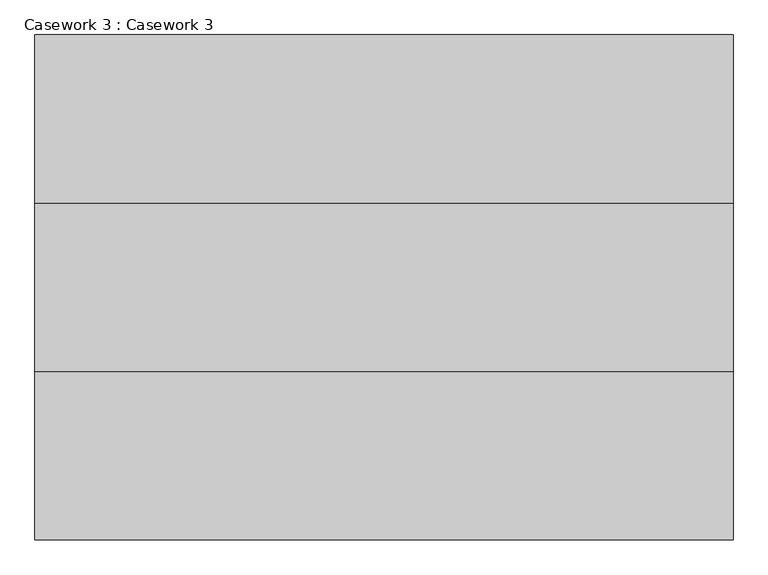
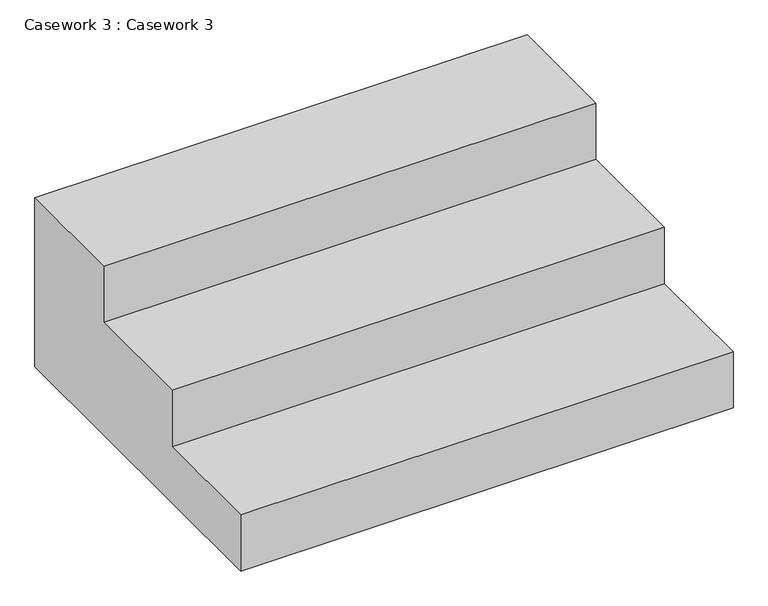
"""IFC4 building model written with IfcOpenShell, lengths in millimetres: furniture geometry, Casework 3 : Casework 3."""

from ifc_helpers import new_model, si_unit, frame, origin, place, context, project, spatial, polyline, outline, extrude, source, transform, mapped, element, save


def casework_3_casework_3_0f97de66(model_context):
    return source(origin(), model_context, "Body", "SweptSolid", [
        extrude(outline(polyline([(-4046.1831926, 2743.2), (-3741.3831926, 2743.2), (-3741.3831926, 2286.0), (-4655.7831926, 2286.0), (-4655.7831926, 2438.4), (-4350.9831926, 2438.4), (-4350.9831926, 2590.8), (-4046.1831926, 2590.8), (-4046.1831926, 2743.2)])), frame((-4879.4781622, 0.0, 0.0), z_axis=(1.0, 0.0, 0.0), x_axis=(0.0, 1.0, 0.0)), (0.0, 0.0, 1.0), 1262.85625),
    ])


if __name__ == "__main__":
    model = new_model("IFC4")
    model_context = context("Model", 3, world=origin())
    ifc_project = project(units=[si_unit("LENGTHUNIT", "METRE", prefix="MILLI")], contexts=[model_context])
    site = spatial("IfcSite", under=ifc_project)
    building = spatial("IfcBuilding", under=site)
    placement = place(None, origin())
    casework_3_casework_3_shape = casework_3_casework_3_0f97de66(model_context)
    element("IfcFurniture", 1, ObjectType="Casework 3 : Casework 3", at=placement, inside=building, context=model_context, shape_type="MappedRepresentation", body=[
        mapped(casework_3_casework_3_shape, transform((0.0, 0.0, 0.0), x_axis=(1.0, 0.0, 0.0), y_axis=(0.0, 1.0, 0.0), z_axis=(0.0, 0.0, 1.0))),
    ])
    save(model, "model.ifc")
